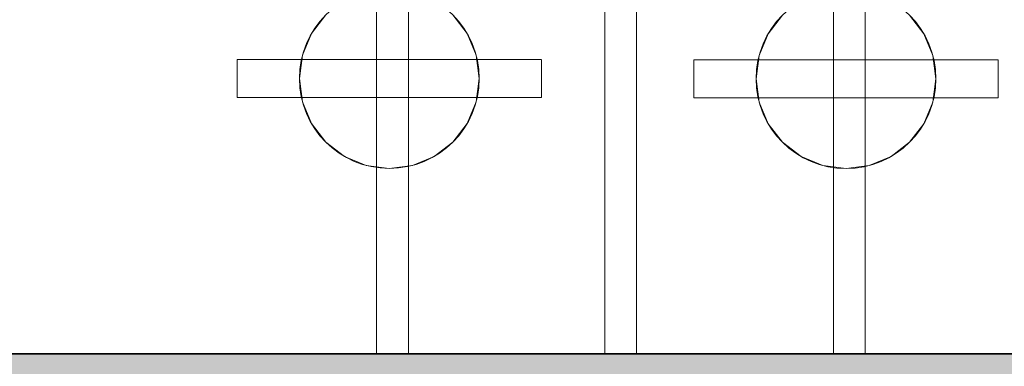
# Model space of a CAD drawing. Units: inches. Extents: x 2696 to 3240, y 1564 to 2310.
# Tile 56 of 76: x 2907.148 to 2916.848, y 2185.477 to 2188.894. Entities that reach past the tile are written whole.
import ezdxf

# ---------------------------------------------------------------- set-up
doc = ezdxf.new("R2010")
doc.units = ezdxf.units.IN
for name, color, linetype, lineweight in [('A-ANNO-DIMS', 3, 'Continuous', 18), ('A-FLOR-FIXT', 8, 'Continuous', 18), ('A-FURN', 251, 'Continuous', 13), ('A-WALL', 7, 'Continuous', 35), ('A-WALL-PATT', 9, 'Continuous', 13)]:
    doc.layers.add(name, color=color, linetype=linetype, lineweight=lineweight)
doc.layers.add('FURNITURE', color=250, linetype='Continuous')
doc.styles.add('TIMES NEW', font='times.ttf')
doc.dimstyles.new('Siddhuu', dxfattribs={"dimtxt": 6, "dimasz": 2.5, "dimexe": 1.25, "dimexo": 0.625, "dimtad": 1, "dimdec": 1, "dimlunit": 4, "dimtxsty": 'TIMES NEW', "dimcen": 2.5, "dimclrd": 256, "dimclre": 1, "dimclrt": 7, "dimadec": 0, "dimazin": 0, "dimtfac": 1, "dimtdec": 1, "dimtmove": 0, "dimatfit": 3, "dimfxl": 1, "dimtolj": 1, "dimlwd": -1, "dimarcsym": 0})

# ---------------------------------------------------------------- blocks, each defined once
blk = doc.blocks.new('A$C1af1f523')
at = {"layer": 'A-FURN'}
for p, q in [((-2.9003, 3.9351), (-2.9003, 0.9365)), ((-2.9003, 3.9351, 0.5), (-2.9003, 0.9365, 0.5)), ((-2.9003, 3.9351), (-2.9003, 3.9351, 0.5)), ((-2.5253, 3.9351), (-2.9003, 3.9351)), ((-2.5253, 3.9351, 0.5), (-2.9003, 3.9351, 0.5)), ((-2.5253, 3.9351), (-2.5253, 0.9365)), ((-2.5253, 3.9351, 0.5), (-2.5253, 0.9365, 0.5)), ((-2.5253, 3.9351), (-2.5253, 3.9351, 0.5)), ((-2.7128, 3.3215), (-2.7128, 3.3215, 0.5)), ((-3.1558, 3.2028), (-3.1558, 3.2028, 0.5)), ((-2.9421, 3.2913), (-2.9421, 3.2913, 0.5)), ((-2.4835, 3.2913), (-2.4835, 3.2913, 0.5)), ((-2.2698, 3.2028), (-2.2698, 3.2028, 0.5)), ((-2.0863, 3.062), (-2.0863, 3.062, 0.5)), ((-1.9455, 2.8785), (-1.9455, 2.8785, 0.5)), ((-1.857, 2.6648), (-1.857, 2.6648, 0.5)), ((0, 2.5605), (-4.2116, 2.5605)), ((0, 2.5605, 0.5), (-4.2116, 2.5605, 0.5)), ((-1.8268, 2.4355), (-1.8268, 2.4355, 0.5)), ((0, 2.248), (-4.2116, 2.248)), ((0, 2.248, 0.5), (-4.2116, 2.248, 0.5)), ((-1.857, 2.2061), (-1.857, 2.2061, 0.5)), ((-1.9455, 1.9924), (-1.9455, 1.9924, 0.5)), ((-2.0863, 1.8089), (-2.0863, 1.8089, 0.5)), ((-3.1558, 1.6681), (-3.1558, 1.6681, 0.5)), ((-2.2698, 1.6681), (-2.2698, 1.6681, 0.5)), ((-2.9421, 1.5796), (-2.9421, 1.5796, 0.5)), ((-2.4835, 1.5796), (-2.4835, 1.5796, 0.5)), ((-2.7128, 1.5494), (-2.7128, 1.5494, 0.5)), ((-2.9003, 0.9365), (-2.9003, 0.9365, 0.5)), ((-2.5253, 0.9365), (-2.8979, 0.9365)), ((-2.5253, 0.9365, 0.5), (-2.8979, 0.9365, 0.5)), ((-2.8979, 0.9365), (-2.8979, 0.9365, 0.5)), ((-2.5253, 0.9365), (-2.5253, 0.9365, 0.5)), ((0, 0.3125), (-6.5015, 0.3125)), ((0, 0.3125, 0.5), (-6.5015, 0.3125, 0.5)), ((0, 0), (-6.5015, 0)), ((0, 0, 0.5), (-6.5015, 0, 0.5)), ((-2.898, -0.5642), (-2.898, -3.5628)), ((-2.898, -0.5642, 0.5), (-2.898, -3.5628, 0.5)), ((-2.898, -0.5642), (-2.898, -0.5642, 0.5)), ((-2.523, -0.5642), (-2.898, -0.5642)), ((-2.523, -0.5642, 0.5), (-2.898, -0.5642, 0.5)), ((-2.523, -0.5642), (-2.523, -3.5628)), ((-2.523, -0.5642, 0.5), (-2.523, -3.5628, 0.5)), ((-2.523, -0.5642), (-2.523, -0.5642, 0.5)), ((-2.9398, -1.208), (-2.9398, -1.208, 0.5)), ((-2.7105, -1.1778), (-2.7105, -1.1778, 0.5)), ((-2.4812, -1.208), (-2.4812, -1.208, 0.5)), ((-3.1535, -1.2965), (-3.1535, -1.2965, 0.5)), ((-2.2675, -1.2965), (-2.2675, -1.2965, 0.5)), ((-2.084, -1.4373), (-2.084, -1.4373, 0.5)), ((-1.9432, -1.6208), (-1.9432, -1.6208, 0.5)), ((-1.8547, -1.8345), (-1.8547, -1.8345, 0.5)), ((0, -1.9388), (-4.2094, -1.9388)), ((0, -1.9388, 0.5), (-4.2094, -1.9388, 0.5)), ((-1.8245, -2.0638), (-1.8245, -2.0638, 0.5)), ((0, -2.2513), (-4.2094, -2.2513)), ((0, -2.2513, 0.5), (-4.2094, -2.2513, 0.5)), ((-1.8547, -2.2931), (-1.8547, -2.2931, 0.5)), ((-1.9432, -2.5068), (-1.9432, -2.5068, 0.5)), ((-2.084, -2.6903), (-2.084, -2.6903, 0.5)), ((-3.1535, -2.8311), (-3.1535, -2.8311, 0.5)), ((-2.2675, -2.8311), (-2.2675, -2.8311, 0.5)), ((-2.9398, -2.9196), (-2.9398, -2.9196, 0.5)), ((-2.7105, -2.9498), (-2.7105, -2.9498, 0.5)), ((-2.4812, -2.9196), (-2.4812, -2.9196, 0.5)), ((-2.898, -3.5628), (-2.898, -3.5628, 0.5)), ((-2.523, -3.5628), (-2.8956, -3.5628)), ((-2.523, -3.5628, 0.5), (-2.8956, -3.5628, 0.5)), ((-2.8956, -3.5628), (-2.8956, -3.5628, 0.5)), ((-2.523, -3.5628), (-2.523, -3.5628, 0.5))]:
    blk.add_line(p, q, dxfattribs=at)
for centre in [(-2.7128, 2.4355), (-2.7128, 2.4355, 0.5), (-2.7105, -2.0638), (-2.7105, -2.0638, 0.5)]:
    blk.add_circle(centre, 0.886, dxfattribs=at)
at = {"layer": 'FURNITURE'}
for p, q in [((0, 2.5605), (0, 2.5605, 0.5)), ((0, 2.248), (0, 2.248, 0.5)), ((0, 0.3125), (0, 0.3125, 0.5)), ((0, 0), (0, 0, 0.5)), ((0, -1.9388), (0, -1.9388, 0.5)), ((0, -2.2513), (0, -2.2513, 0.5))]:
    blk.add_line(p, q, dxfattribs=at)
at = {"layer": 'A-FURN'}
mesh = blk.add_polyface(dxfattribs=at)
corners = [(-2.9003, 0.9365, 0.5), (-2.9003, 3.9351), (-2.9003, 0.9365), (-2.9003, 3.9351, 0.5)]
mesh.append_faces([[corners[k] for k in face] for face in [(2, 1, 0), (3, 0, 1)]], dxfattribs={"vtx1": -1})
mesh = blk.add_polyface(dxfattribs=at)
corners = [(-2.5253, 3.9351, 0.5), (-2.9003, 3.9351), (-2.9003, 3.9351, 0.5), (-2.5253, 3.9351)]
mesh.append_faces([[corners[k] for k in face] for face in [(2, 1, 0), (3, 0, 1)]], dxfattribs={"vtx1": -1})
mesh = blk.add_polyface(dxfattribs=at)
corners = [(-2.5253, 0.9365, 0.5), (-2.5253, 3.9351), (-2.5253, 0.9365), (-2.5253, 3.9351, 0.5)]
mesh.append_faces([[corners[k] for k in face] for face in [(2, 1, 0), (3, 0, 1)]], dxfattribs={"vtx1": -1})
mesh = blk.add_polyface(dxfattribs=at)
corners = [(-2.7128, 3.3215), (-2.9421, 3.2913, 0.5), (-2.9421, 3.2913), (-2.7128, 3.3215, 0.5)]
mesh.append_faces([[corners[k] for k in face] for face in [(2, 1, 0), (3, 0, 1)]], dxfattribs={"vtx1": -1})
mesh = blk.add_polyface(dxfattribs=at)
corners = [(-2.4835, 3.2913), (-2.7128, 3.3215, 0.5), (-2.7128, 3.3215), (-2.4835, 3.2913, 0.5)]
mesh.append_faces([[corners[k] for k in face] for face in [(2, 1, 0), (3, 0, 1)]], dxfattribs={"vtx1": -1})
mesh = blk.add_polyface(dxfattribs=at)
corners = [(-3.1558, 3.2028), (-3.3393, 3.062, 0.5), (-3.3393, 3.062), (-3.1558, 3.2028, 0.5)]
mesh.append_faces([[corners[k] for k in face] for face in [(2, 1, 0), (3, 0, 1)]], dxfattribs={"vtx1": -1})
mesh = blk.add_polyface(dxfattribs=at)
corners = [(-2.9421, 3.2913), (-3.1558, 3.2028, 0.5), (-3.1558, 3.2028), (-2.9421, 3.2913, 0.5)]
mesh.append_faces([[corners[k] for k in face] for face in [(2, 1, 0), (3, 0, 1)]], dxfattribs={"vtx1": -1})
mesh = blk.add_polyface(dxfattribs=at)
corners = [(-2.2698, 3.2028), (-2.4835, 3.2913, 0.5), (-2.4835, 3.2913), (-2.2698, 3.2028, 0.5)]
mesh.append_faces([[corners[k] for k in face] for face in [(2, 1, 0), (3, 0, 1)]], dxfattribs={"vtx1": -1})
mesh = blk.add_polyface(dxfattribs=at)
corners = [(-2.0863, 3.062), (-2.2698, 3.2028, 0.5), (-2.2698, 3.2028), (-2.0863, 3.062, 0.5)]
mesh.append_faces([[corners[k] for k in face] for face in [(2, 1, 0), (3, 0, 1)]], dxfattribs={"vtx1": -1})
mesh = blk.add_polyface(dxfattribs=at)
corners = [(-1.9455, 2.8785, 0.5), (-2.0863, 3.062), (-1.9455, 2.8785), (-2.0863, 3.062, 0.5)]
mesh.append_faces([[corners[k] for k in face] for face in [(2, 1, 0), (3, 0, 1)]], dxfattribs={"vtx1": -1})
mesh = blk.add_polyface(dxfattribs=at)
corners = [(-1.857, 2.6648, 0.5), (-1.9455, 2.8785), (-1.857, 2.6648), (-1.9455, 2.8785, 0.5)]
mesh.append_faces([[corners[k] for k in face] for face in [(2, 1, 0), (3, 0, 1)]], dxfattribs={"vtx1": -1})
mesh = blk.add_polyface(dxfattribs=at)
corners = [(-1.8268, 2.4355, 0.5), (-1.857, 2.6648), (-1.8268, 2.4355), (-1.857, 2.6648, 0.5)]
mesh.append_faces([[corners[k] for k in face] for face in [(2, 1, 0), (3, 0, 1)]], dxfattribs={"vtx1": -1})
mesh = blk.add_polyface(dxfattribs=at)
corners = [(0, 2.5605, 0.5), (-4.2116, 2.5605), (-4.2116, 2.5605, 0.5), (0, 2.5605)]
mesh.append_faces([[corners[k] for k in face] for face in [(2, 1, 0), (3, 0, 1)]], dxfattribs={"vtx1": -1})
mesh = blk.add_polyface(dxfattribs=at)
corners = [(-1.857, 2.2061, 0.5), (-1.8268, 2.4355), (-1.857, 2.2061), (-1.8268, 2.4355, 0.5)]
mesh.append_faces([[corners[k] for k in face] for face in [(2, 1, 0), (3, 0, 1)]], dxfattribs={"vtx1": -1})
mesh = blk.add_polyface(dxfattribs=at)
corners = [(0, 2.248, 0.5), (-4.2116, 2.248), (-4.2116, 2.248, 0.5), (0, 2.248)]
mesh.append_faces([[corners[k] for k in face] for face in [(2, 1, 0), (3, 0, 1)]], dxfattribs={"vtx1": -1})
mesh = blk.add_polyface(dxfattribs=at)
corners = [(-1.9455, 1.9924, 0.5), (-1.857, 2.2061), (-1.9455, 1.9924), (-1.857, 2.2061, 0.5)]
mesh.append_faces([[corners[k] for k in face] for face in [(2, 1, 0), (3, 0, 1)]], dxfattribs={"vtx1": -1})
mesh = blk.add_polyface(dxfattribs=at)
corners = [(-2.0863, 1.8089, 0.5), (-1.9455, 1.9924), (-2.0863, 1.8089), (-1.9455, 1.9924, 0.5)]
mesh.append_faces([[corners[k] for k in face] for face in [(2, 1, 0), (3, 0, 1)]], dxfattribs={"vtx1": -1})
mesh = blk.add_polyface(dxfattribs=at)
corners = [(-3.1558, 1.6681, 0.5), (-3.3393, 1.8089), (-3.3393, 1.8089, 0.5), (-3.1558, 1.6681)]
mesh.append_faces([[corners[k] for k in face] for face in [(2, 1, 0), (3, 0, 1)]], dxfattribs={"vtx1": -1})
mesh = blk.add_polyface(dxfattribs=at)
corners = [(-2.0863, 1.8089, 0.5), (-2.2698, 1.6681), (-2.2698, 1.6681, 0.5), (-2.0863, 1.8089)]
mesh.append_faces([[corners[k] for k in face] for face in [(2, 1, 0), (3, 0, 1)]], dxfattribs={"vtx1": -1})
mesh = blk.add_polyface(dxfattribs=at)
corners = [(-2.9421, 1.5796, 0.5), (-3.1558, 1.6681), (-3.1558, 1.6681, 0.5), (-2.9421, 1.5796)]
mesh.append_faces([[corners[k] for k in face] for face in [(2, 1, 0), (3, 0, 1)]], dxfattribs={"vtx1": -1})
mesh = blk.add_polyface(dxfattribs=at)
corners = [(-2.2698, 1.6681, 0.5), (-2.4835, 1.5796), (-2.4835, 1.5796, 0.5), (-2.2698, 1.6681)]
mesh.append_faces([[corners[k] for k in face] for face in [(2, 1, 0), (3, 0, 1)]], dxfattribs={"vtx1": -1})
mesh = blk.add_polyface(dxfattribs=at)
corners = [(-2.7128, 1.5494, 0.5), (-2.9421, 1.5796), (-2.9421, 1.5796, 0.5), (-2.7128, 1.5494)]
mesh.append_faces([[corners[k] for k in face] for face in [(2, 1, 0), (3, 0, 1)]], dxfattribs={"vtx1": -1})
mesh = blk.add_polyface(dxfattribs=at)
corners = [(-2.4835, 1.5796, 0.5), (-2.7128, 1.5494), (-2.7128, 1.5494, 0.5), (-2.4835, 1.5796)]
mesh.append_faces([[corners[k] for k in face] for face in [(2, 1, 0), (3, 0, 1)]], dxfattribs={"vtx1": -1})
mesh = blk.add_polyface(dxfattribs=at)
corners = [(-2.5253, 0.9365, 0.5), (-2.8979, 0.9365), (-2.8979, 0.9365, 0.5), (-2.5253, 0.9365)]
mesh.append_faces([[corners[k] for k in face] for face in [(2, 1, 0), (3, 0, 1)]], dxfattribs={"vtx1": -1})
mesh = blk.add_polyface(dxfattribs=at)
corners = [(0, 0.3125, 0.5), (-6.5015, 0.3125), (-6.5015, 0.3125, 0.5), (0, 0.3125)]
mesh.append_faces([[corners[k] for k in face] for face in [(2, 1, 0), (3, 0, 1)]], dxfattribs={"vtx1": -1})
mesh = blk.add_polyface(dxfattribs=at)
corners = [(0, 0, 0.5), (-6.5015, 0), (-6.5015, 0, 0.5), (0, 0)]
mesh.append_faces([[corners[k] for k in face] for face in [(2, 1, 0), (3, 0, 1)]], dxfattribs={"vtx1": -1})
mesh = blk.add_polyface(dxfattribs=at)
corners = [(-2.898, -3.5628, 0.5), (-2.898, -0.5642), (-2.898, -3.5628), (-2.898, -0.5642, 0.5)]
mesh.append_faces([[corners[k] for k in face] for face in [(2, 1, 0), (3, 0, 1)]], dxfattribs={"vtx1": -1})
mesh = blk.add_polyface(dxfattribs=at)
corners = [(-2.523, -0.5642, 0.5), (-2.898, -0.5642), (-2.898, -0.5642, 0.5), (-2.523, -0.5642)]
mesh.append_faces([[corners[k] for k in face] for face in [(2, 1, 0), (3, 0, 1)]], dxfattribs={"vtx1": -1})
mesh = blk.add_polyface(dxfattribs=at)
corners = [(-2.523, -3.5628, 0.5), (-2.523, -0.5642), (-2.523, -3.5628), (-2.523, -0.5642, 0.5)]
mesh.append_faces([[corners[k] for k in face] for face in [(2, 1, 0), (3, 0, 1)]], dxfattribs={"vtx1": -1})
mesh = blk.add_polyface(dxfattribs=at)
corners = [(-2.9398, -1.208), (-3.1535, -1.2965, 0.5), (-3.1535, -1.2965), (-2.9398, -1.208, 0.5)]
mesh.append_faces([[corners[k] for k in face] for face in [(2, 1, 0), (3, 0, 1)]], dxfattribs={"vtx1": -1})
mesh = blk.add_polyface(dxfattribs=at)
corners = [(-2.7105, -1.1778), (-2.9398, -1.208, 0.5), (-2.9398, -1.208), (-2.7105, -1.1778, 0.5)]
mesh.append_faces([[corners[k] for k in face] for face in [(2, 1, 0), (3, 0, 1)]], dxfattribs={"vtx1": -1})
mesh = blk.add_polyface(dxfattribs=at)
corners = [(-2.4812, -1.208), (-2.7105, -1.1778, 0.5), (-2.7105, -1.1778), (-2.4812, -1.208, 0.5)]
mesh.append_faces([[corners[k] for k in face] for face in [(2, 1, 0), (3, 0, 1)]], dxfattribs={"vtx1": -1})
mesh = blk.add_polyface(dxfattribs=at)
corners = [(-2.2675, -1.2965), (-2.4812, -1.208, 0.5), (-2.4812, -1.208), (-2.2675, -1.2965, 0.5)]
mesh.append_faces([[corners[k] for k in face] for face in [(2, 1, 0), (3, 0, 1)]], dxfattribs={"vtx1": -1})
mesh = blk.add_polyface(dxfattribs=at)
corners = [(-3.1535, -1.2965), (-3.337, -1.4373, 0.5), (-3.337, -1.4373), (-3.1535, -1.2965, 0.5)]
mesh.append_faces([[corners[k] for k in face] for face in [(2, 1, 0), (3, 0, 1)]], dxfattribs={"vtx1": -1})
mesh = blk.add_polyface(dxfattribs=at)
corners = [(-2.084, -1.4373), (-2.2675, -1.2965, 0.5), (-2.2675, -1.2965), (-2.084, -1.4373, 0.5)]
mesh.append_faces([[corners[k] for k in face] for face in [(2, 1, 0), (3, 0, 1)]], dxfattribs={"vtx1": -1})
mesh = blk.add_polyface(dxfattribs=at)
corners = [(-1.9432, -1.6208, 0.5), (-2.084, -1.4373), (-1.9432, -1.6208), (-2.084, -1.4373, 0.5)]
mesh.append_faces([[corners[k] for k in face] for face in [(2, 1, 0), (3, 0, 1)]], dxfattribs={"vtx1": -1})
mesh = blk.add_polyface(dxfattribs=at)
corners = [(-1.8547, -1.8345, 0.5), (-1.9432, -1.6208), (-1.8547, -1.8345), (-1.9432, -1.6208, 0.5)]
mesh.append_faces([[corners[k] for k in face] for face in [(2, 1, 0), (3, 0, 1)]], dxfattribs={"vtx1": -1})
mesh = blk.add_polyface(dxfattribs=at)
corners = [(-1.8245, -2.0638, 0.5), (-1.8547, -1.8345), (-1.8245, -2.0638), (-1.8547, -1.8345, 0.5)]
mesh.append_faces([[corners[k] for k in face] for face in [(2, 1, 0), (3, 0, 1)]], dxfattribs={"vtx1": -1})
mesh = blk.add_polyface(dxfattribs=at)
corners = [(0, -1.9388, 0.5), (-4.2094, -1.9388), (-4.2094, -1.9388, 0.5), (0, -1.9388)]
mesh.append_faces([[corners[k] for k in face] for face in [(2, 1, 0), (3, 0, 1)]], dxfattribs={"vtx1": -1})
mesh = blk.add_polyface(dxfattribs=at)
corners = [(-1.8547, -2.2931, 0.5), (-1.8245, -2.0638), (-1.8547, -2.2931), (-1.8245, -2.0638, 0.5)]
mesh.append_faces([[corners[k] for k in face] for face in [(2, 1, 0), (3, 0, 1)]], dxfattribs={"vtx1": -1})
mesh = blk.add_polyface(dxfattribs=at)
corners = [(0, -2.2513, 0.5), (-4.2094, -2.2513), (-4.2094, -2.2513, 0.5), (0, -2.2513)]
mesh.append_faces([[corners[k] for k in face] for face in [(2, 1, 0), (3, 0, 1)]], dxfattribs={"vtx1": -1})
mesh = blk.add_polyface(dxfattribs=at)
corners = [(-1.9432, -2.5068, 0.5), (-1.8547, -2.2931), (-1.9432, -2.5068), (-1.8547, -2.2931, 0.5)]
mesh.append_faces([[corners[k] for k in face] for face in [(2, 1, 0), (3, 0, 1)]], dxfattribs={"vtx1": -1})
mesh = blk.add_polyface(dxfattribs=at)
corners = [(-2.084, -2.6903, 0.5), (-1.9432, -2.5068), (-2.084, -2.6903), (-1.9432, -2.5068, 0.5)]
mesh.append_faces([[corners[k] for k in face] for face in [(2, 1, 0), (3, 0, 1)]], dxfattribs={"vtx1": -1})
mesh = blk.add_polyface(dxfattribs=at)
corners = [(-3.1535, -2.8311, 0.5), (-3.337, -2.6903), (-3.337, -2.6903, 0.5), (-3.1535, -2.8311)]
mesh.append_faces([[corners[k] for k in face] for face in [(2, 1, 0), (3, 0, 1)]], dxfattribs={"vtx1": -1})
mesh = blk.add_polyface(dxfattribs=at)
corners = [(-2.084, -2.6903, 0.5), (-2.2675, -2.8311), (-2.2675, -2.8311, 0.5), (-2.084, -2.6903)]
mesh.append_faces([[corners[k] for k in face] for face in [(2, 1, 0), (3, 0, 1)]], dxfattribs={"vtx1": -1})
mesh = blk.add_polyface(dxfattribs=at)
corners = [(-2.9398, -2.9196, 0.5), (-3.1535, -2.8311), (-3.1535, -2.8311, 0.5), (-2.9398, -2.9196)]
mesh.append_faces([[corners[k] for k in face] for face in [(2, 1, 0), (3, 0, 1)]], dxfattribs={"vtx1": -1})
mesh = blk.add_polyface(dxfattribs=at)
corners = [(-2.2675, -2.8311, 0.5), (-2.4812, -2.9196), (-2.4812, -2.9196, 0.5), (-2.2675, -2.8311)]
mesh.append_faces([[corners[k] for k in face] for face in [(2, 1, 0), (3, 0, 1)]], dxfattribs={"vtx1": -1})
mesh = blk.add_polyface(dxfattribs=at)
corners = [(-2.7105, -2.9498, 0.5), (-2.9398, -2.9196), (-2.9398, -2.9196, 0.5), (-2.7105, -2.9498)]
mesh.append_faces([[corners[k] for k in face] for face in [(2, 1, 0), (3, 0, 1)]], dxfattribs={"vtx1": -1})
mesh = blk.add_polyface(dxfattribs=at)
corners = [(-2.4812, -2.9196, 0.5), (-2.7105, -2.9498), (-2.7105, -2.9498, 0.5), (-2.4812, -2.9196)]
mesh.append_faces([[corners[k] for k in face] for face in [(2, 1, 0), (3, 0, 1)]], dxfattribs={"vtx1": -1})
mesh = blk.add_polyface(dxfattribs=at)
corners = [(-2.523, -3.5628, 0.5), (-2.8956, -3.5628), (-2.8956, -3.5628, 0.5), (-2.523, -3.5628)]
mesh.append_faces([[corners[k] for k in face] for face in [(2, 1, 0), (3, 0, 1)]], dxfattribs={"vtx1": -1})
blk = doc.blocks.new('*D59')
at = {"layer": 'A-ANNO-DIMS', "color": 1, "lineweight": -2, "transparency": 16777216}
for p, q in [((2884.7088, 1740.8261), (2884.7088, 2298.4511)), ((2956.7088, 1740.8261), (2956.7088, 2298.4511))]:
    blk.add_line(p, q, dxfattribs=at)
at = {"layer": 'A-ANNO-DIMS', "transparency": 16777216}
blk.add_line((2887.2088, 2297.2011), (2954.2088, 2297.2011), dxfattribs=at)
for points in [[(2887.2088, 2297.6178), (2887.2088, 2296.7844), (2884.7088, 2297.2011)], [(2954.2088, 2297.6178), (2954.2088, 2296.7844), (2956.7088, 2297.2011)]]:
    blk.add_solid(points, dxfattribs=at)
at = {"layer": 'Defpoints', "color": 0, "transparency": 16777216}
for p in [(2956.7088, 2297.2011), (2884.7088, 1740.2011), (2956.7088, 1740.2011)]:
    blk.add_point(p, dxfattribs=at)
at = {"layer": 'A-ANNO-DIMS', "color": 7, "transparency": 16777216, "insert": (2920.7088, 2300.878), "char_height": 6, "attachment_point": 5, "style": 'TIMES NEW'}
blk.add_mtext('\\A1;6\'-0"', dxfattribs=at)
blk = doc.blocks.new('*D64')
at = {"layer": 'A-ANNO-DIMS', "color": 1, "lineweight": -2, "transparency": 16777216}
for p, q in [((3073.0838, 2206.7011), (2709.3614, 2206.7011)), ((3068.5838, 1989.2011), (2709.3614, 1989.2011))]:
    blk.add_line(p, q, dxfattribs=at)
at = {"layer": 'A-ANNO-DIMS', "transparency": 16777216}
blk.add_line((2710.6114, 1991.7011), (2710.6114, 2204.2011), dxfattribs=at)
for points in [[(2710.1947, 2204.2011), (2711.0281, 2204.2011), (2710.6114, 2206.7011)], [(2710.1947, 1991.7011), (2711.0281, 1991.7011), (2710.6114, 1989.2011)]]:
    blk.add_solid(points, dxfattribs=at)
at = {"layer": 'Defpoints', "color": 0, "transparency": 16777216}
for p in [(2710.6114, 2206.7011), (3073.7088, 2206.7011), (3069.2088, 1989.2011)]:
    blk.add_point(p, dxfattribs=at)
at = {"layer": 'A-ANNO-DIMS', "color": 7, "transparency": 16777216, "insert": (2706.8501, 2097.9511), "char_height": 6, "attachment_point": 5, "rotation": 90, "style": 'TIMES NEW'}
blk.add_mtext('\\A1;18\'-1 1/2"', dxfattribs=at)

msp = doc.modelspace()

# ---------------------------------------------------------------- hatches: boundary and pattern name
at = {"layer": 'A-WALL-PATT', "transparency": 33554556}
h = msp.add_hatch(color=256, dxfattribs=at)
h.dxf.hatch_style = 1
h.paths.add_polyline_path([(2879.1114, 2253.2011), (2905.9101, 2253.2011), (2905.9101, 2262.2011), (2841.889, 2262.2011), (2841.889, 2253.2011), (2870.1114, 2253.2011), (2870.1114, 2176.6011), (2965.7088, 2176.6011), (2965.7088, 2206.7011), (2973.5828, 2206.7011), (2973.5828, 2215.7011), (2965.7088, 2215.7011), (2965.7088, 2262.2011), (2929.9101, 2262.2011), (2929.9101, 2253.2011), (2956.7088, 2253.2011), (2956.7088, 2185.6011), (2879.1114, 2185.6011)])
h.paths.add_polyline_path([(2782.8338, 2262.2011), (2745.6114, 2262.2011), (2745.6114, 2228.7287), (2754.6114, 2228.7287), (2754.6114, 2253.2011), (2782.8338, 2253.2011)])
h.paths.add_polyline_path([(2754.6114, 2136.2011), (2965.7088, 2136.2011), (2965.7088, 2145.2011), (2879.1114, 2145.2011), (2879.1114, 2147.0735), (2877.3397, 2147.0735), (2870.1114, 2147.0735), (2870.1114, 2145.2011), (2754.6114, 2145.2011), (2754.6114, 2169.6735), (2745.6114, 2169.6735), (2745.6114, 2000.2011), (2754.6114, 2000.2011), (2754.6114, 2019.2011), (2849.0828, 2019.2011), (2849.0828, 2023.7011), (2841.2088, 2023.7011), (2841.2088, 2051.8271), (2836.7088, 2051.8271), (2836.7088, 2023.7011), (2754.6114, 2023.7011), (2754.6114, 2091.2011), (2836.7088, 2091.2011), (2836.7088, 2087.8271), (2841.2088, 2087.8271), (2841.2088, 2095.7011), (2754.6114, 2095.7011)])
h.paths.add_polyline_path([(2965.7088, 2136.2011), (2956.7088, 2136.2011), (2956.7088, 2023.7011), (2885.0828, 2023.7011), (2885.0828, 2019.2011), (2956.7088, 2019.2011), (2956.7088, 1950.5751), (2965.7088, 1950.5751), (2965.7088, 1980.2011), (2973.5828, 1980.2011), (2973.5828, 1989.2011), (2965.7088, 1989.2011)])
h.paths.add_polyline_path([(2754.6114, 1906.7011), (2880.2088, 1906.7011), (2884.7088, 1906.7011), (2956.7088, 1906.7011), (2956.7088, 1792.7011), (2944.7088, 1792.7011), (2944.7088, 1783.7011), (2956.7088, 1783.7011), (2956.7088, 1740.2011), (2884.7088, 1740.2011), (2884.7088, 1783.7011), (2896.7088, 1783.7011), (2896.7088, 1792.7011), (2884.7088, 1792.7011), (2884.7088, 1846.7011), (2880.2088, 1846.7011), (2880.2088, 1740.2011), (2754.6114, 1740.2011), (2754.6114, 1777.2011), (2745.6114, 1777.2011), (2745.6114, 1692.7011), (2754.6114, 1692.7011), (2754.6114, 1731.2011), (2956.7088, 1731.2011), (2956.7088, 1723.3271), (2965.7088, 1723.3271), (2965.7088, 1884.2011), (2973.5828, 1884.2011), (2973.5828, 1893.2011), (2965.7088, 1893.2011), (2965.7088, 1914.5751), (2956.7088, 1914.5751), (2956.7088, 1911.2011), (2754.6114, 1911.2011), (2754.6114, 1930.2011), (2745.6114, 1930.2011), (2745.6114, 1817.2011), (2754.6114, 1817.2011), (2754.6114, 1854.2011), (2826.6114, 1854.2011), (2826.6114, 1868.8271), (2822.1114, 1868.8271), (2822.1114, 1858.7011), (2754.6114, 1858.7011)])
h.paths.add_polyline_path([(2965.7088, 1656.2011), (3008.2374, 1656.2011), (3008.2374, 1665.2011), (2965.7088, 1665.2011), (2965.7088, 1693.3271), (2956.7088, 1693.3271), (2956.7088, 1686.2011), (2934.5828, 1686.2011), (2934.5828, 1681.7011), (2956.7088, 1681.7011), (2956.7088, 1614.2011), (2896.7088, 1614.2011), (2896.7088, 1681.7011), (2904.5828, 1681.7011), (2904.5828, 1686.2011), (2892.2088, 1686.2011), (2892.2088, 1614.2011), (2858.4101, 1614.2011), (2858.4101, 1605.2011), (2965.7088, 1605.2011)])
h.paths.add_polyline_path([(2788.4101, 1614.2011), (2754.6114, 1614.2011), (2754.6114, 1652.7011), (2745.6114, 1652.7011), (2745.6114, 1605.2011), (2788.4101, 1605.2011)])
h.paths.add_polyline_path([(3199.6114, 1633.0476), (3190.6114, 1633.0476), (3190.6114, 1614.2011), (3082.6114, 1614.2011), (3082.6114, 1665.2011), (3070.2374, 1665.2011), (3070.2374, 1656.2011), (3078.1114, 1656.2011), (3078.1114, 1605.2011), (3199.6114, 1605.2011)])
h.paths.add_polyline_path([(3199.6114, 1702.0476), (3190.6114, 1702.0476), (3190.6114, 1699.7011), (3106.6114, 1699.7011), (3106.6114, 1747.7011), (3190.6114, 1747.7011), (3190.6114, 1752.2011), (3082.6114, 1752.2011), (3082.6114, 1760.0751), (3078.1114, 1760.0751), (3078.1114, 1747.7011), (3102.1114, 1747.7011), (3102.1114, 1699.7011), (3078.1114, 1699.7011), (3078.1114, 1695.2011), (3190.6114, 1695.2011), (3190.6114, 1676.3546), (3199.6114, 1676.3546)])
h.paths.add_polyline_path([(3199.6114, 1783.2011), (3190.6114, 1783.2011), (3190.6114, 1745.3546), (3199.6114, 1745.3546)])
h.paths.add_polyline_path([(3082.6114, 1884.2011), (3190.6114, 1884.2011), (3190.6114, 1853.2011), (3199.6114, 1853.2011), (3199.6114, 1901.7011), (3190.6114, 1901.7011), (3190.6114, 1893.2011), (3005.5828, 1893.2011), (3005.5828, 1891.2811), (3005.5828, 1884.2011), (3078.1114, 1884.2011), (3078.1114, 1792.0751), (3082.6114, 1792.0751)])
h.paths.add_polyline_path([(3199.6114, 1994.7011), (3190.6114, 1994.7011), (3190.6114, 1989.2011), (3073.7088, 1989.2011), (3073.7088, 2034.2011), (3069.2088, 2034.2011), (3069.2088, 1989.2011), (3005.5828, 1989.2011), (3005.5828, 1980.2011), (3190.6114, 1980.2011), (3190.6114, 1971.7011), (3199.6114, 1971.7011)])
h.paths.add_polyline_path([(3199.6114, 2155.2011), (3190.6114, 2155.2011), (3190.6114, 2064.7011), (3199.6114, 2064.7011)])
h.paths.add_polyline_path([(3190.6114, 2074.7011), (3106.6114, 2074.7011), (3106.6114, 2122.7011), (3190.6114, 2122.7011), (3190.6114, 2127.2011), (3082.7088, 2127.2011), (3082.7088, 2135.0751), (3073.7088, 2135.0751), (3073.7088, 2122.7011), (3102.1114, 2122.7011), (3102.1114, 2074.7011), (3069.2088, 2074.7011), (3069.2088, 2070.2011), (3190.6114, 2070.2011)])
h.paths.add_polyline_path([(3082.7088, 2253.2011), (3190.6114, 2253.2011), (3190.6114, 2225.2011), (3199.6114, 2225.2011), (3199.6114, 2262.2011), (3073.7088, 2262.2011), (3073.7088, 2215.7011), (3035.5828, 2215.7011), (3035.5828, 2206.7011), (3073.7088, 2206.7011), (3073.7088, 2171.0751), (3082.7088, 2171.0751)])

# ---------------------------------------------------------------- linework, layer by layer
at = {"layer": 'A-WALL'}
msp.add_line((2879.1114, 2185.6011), (2956.7088, 2185.6011), dxfattribs=at)

# ---------------------------------------------------------------- block references
at = {"layer": 'A-FLOR-FIXT', "xscale": -1, "rotation": 90}
msp.add_blockref('A$C1af1f523', (2913.2252, 2185.6011), dxfattribs=at)

# ---------------------------------------------------------------- dimensions: what is measured, and where the dimension line sits
at = {"layer": 'A-ANNO-DIMS'}
dim = msp.add_linear_dim(base=(2956.7088, 2297.2011), p1=(2884.7088, 1740.2011), p2=(2956.7088, 1740.2011), dimstyle='Siddhuu', override={"dimdec": 1, "dimlfac": 1, "dimrnd": 0, "dimzin": 1, "dimdsep": 46, "dimlunit": 4, "dimfrac": 2}, dxfattribs=at)
dim.commit()
dim.dimension.update_dxf_attribs({"geometry": '*D59', "text_midpoint": (2920.7088, 2300.878)})
dim = msp.add_linear_dim(base=(2710.6114, 2206.7011), p1=(3069.2088, 1989.2011), p2=(3073.7088, 2206.7011), angle=90, dimstyle='Siddhuu', override={"dimdec": 1, "dimlfac": 1, "dimrnd": 0, "dimzin": 1, "dimdsep": 46, "dimlunit": 4, "dimfrac": 2}, dxfattribs=at)
dim.commit()
dim.dimension.update_dxf_attribs({"geometry": '*D64', "text_midpoint": (2706.8501, 2097.9511)})

doc.saveas('drawing.dxf')
